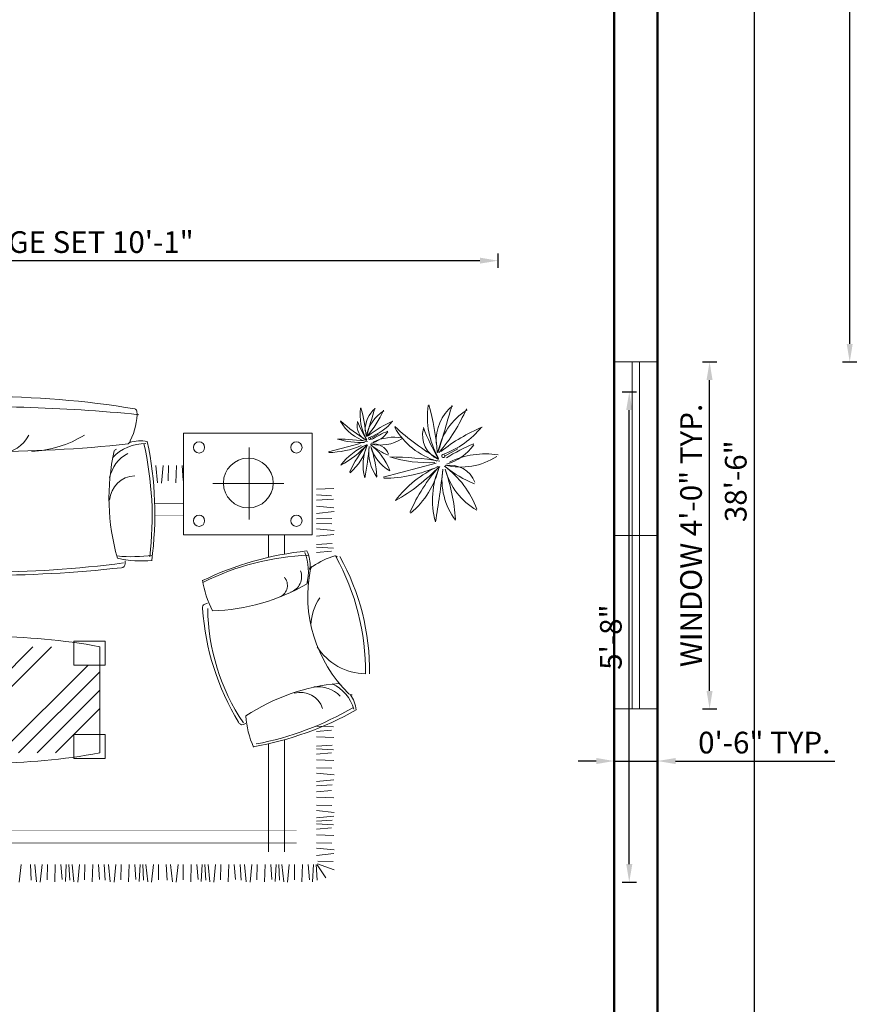
# Model space of a CAD drawing. Units: inches. Extents: x 1961 to 3038, y 800 to 1438.
# Tile 10 of 13: x 2920 to 3038, y 1012 to 1148. Entities that reach past the tile are written whole.
import ezdxf

# ---------------------------------------------------------------- set-up
doc = ezdxf.new("R2010")
doc.units = ezdxf.units.IN
for name, color, linetype, lineweight in [('A-ANNO-DIMS', 2, 'Continuous', 18), ('A-FURN', 8, 'Continuous', 18), ('A-GLAZ', 4, 'Continuous', 18), ('A-WALL', 7, 'Continuous', 50)]:
    doc.layers.add(name, color=color, linetype=linetype, lineweight=lineweight)
doc.styles.get("Standard").update_dxf_attribs({"font": 'arial.ttf'})
doc.dimstyles.new('ISO-25', dxfattribs={"dimtxt": 3, "dimasz": 2.5, "dimexe": 1, "dimexo": 1, "dimtad": 1, "dimdec": 4, "dimlunit": 4, "dimtxsty": 'Standard', "dimcen": 2.5, "dimadec": 0, "dimazin": 0, "dimtfac": 1, "dimtdec": 4, "dimtmove": 0, "dimatfit": 3, "dimfxl": 1, "dimfxlon": 1, "dimarcsym": 0})

# ---------------------------------------------------------------- blocks, each defined once
blk = doc.blocks.new('A$C28C76B35')
for p, q in [((630.8, 2791.1), (1149.7, 2272.2)), ((630.8, 2701.3), (1149.7, 2182.4)), ((630.8, 2431.9), (1059.7, 2003)), ((86.3, 2330.2, -715.1), (0, 2338.9, -715.1)), ((630.8, 2342.1), (1027.2, 1945.7)), ((86.3, 2263.8, -715.1), (1.4, 2255.2, -715.1)), ((86.3, 2285, -715.1), (10.1, 2280.7, -715.1)), ((86.3, 2227.8, -715.1), (0, 2236.5, -715.1)), ((630.8, 2252.3), (937.3, 1945.7)), ((86.3, 2163, -715.1), (1.4, 2165.9, -715.1)), ((86.3, 2201.9, -715.1), (11.5, 2203.3, -715.1)), ((86.3, 2135.7, -715.1), (13, 2129.9, -715.1)), ((630.8, 2162.5), (720.3, 2073)), ((86.3, 2080.9, -715.1), (1.4, 2072.3, -715.1)), ((86.3, 2109.7, -715.1), (2.9, 2114, -715.1)), ((86.3, 2096.8, -715.1), (10.1, 2092.4, -715.1)), ((720.8, 2072.5), (847.5, 1945.7)), ((86.3, 2044.9, -715.1), (0, 2053.6, -715.1)), ((86.3, 2019, -715.1), (11.5, 2020.4, -715.1)), ((86.3, 1980.1, -715.1), (1.4, 1983, -715.1)), ((86.3, 1924.1, -715.1), (10.1, 1919.7, -715.1)), ((86.3, 1952.7, -715.1), (13, 1947, -715.1)), ((1149.7, 1945.7), (630.8, 1945.7)), ((86.3, 1866.9, -715.1), (0, 1875.6, -715.1)), ((86.3, 1902.9, -715.1), (1.4, 1894.3, -715.1)), ((86.3, 1841, -715.1), (11.5, 1842.4, -715.1)), ((86.3, 1802.1, -715.1), (1.4, 1805, -715.1)), ((1569.5, 1821.1, -2545.7), (1554.2, 1821.1, -2545.7)), ((86.3, 1748.8, -715.1), (2.9, 1753.1, -715.1)), ((86.3, 1735.9, -715.1), (10.1, 1731.5, -715.1)), ((86.3, 1774.7, -715.1), (13, 1769, -715.1)), ((86.3, 1684, -715.1), (0, 1692.6, -715.1)), ((86.3, 1720, -715.1), (1.4, 1711.4, -715.1)), ((86.3, 1658.1, -715.1), (11.5, 1659.5, -715.1)), ((2034.4, 1635.7, -715.1), (1948.1, 1644.4, -715.1)), ((2034.4, 1671.7, -715.1), (1949.5, 1663.1, -715.1)), ((86.3, 1599.5, -715.1), (1.4, 1590.9, -715.1)), ((86.3, 1620.7, -715.1), (10.1, 1616.4, -715.1)), ((2034.4, 1609.8, -715.1), (1959.6, 1611.2, -715.1)), ((86.3, 1563.5, -715.1), (0, 1572.2, -715.1)), ((86.3, 1537.6, -715.1), (11.5, 1539, -715.1)), ((2034.4, 1570.9, -715.1), (1949.5, 1573.8, -715.1)), ((2034.4, 1543.6, -715.1), (1961, 1537.8, -715.1)), ((86.3, 1498.7, -715.1), (1.4, 1501.6, -715.1)), ((86.3, 1445.4, -715.1), (2.9, 1449.8, -715.1)), ((86.3, 1471.4, -715.1), (13, 1465.6, -715.1)), ((86.3, 1416.6, -715.1), (1.4, 1408, -715.1)), ((86.3, 1432.5, -715.1), (10.1, 1428.1, -715.1)), ((1361.7, 1420, -2396.1), (1357.7, 1432.5, -2396.1)), ((86.3, 1380.6, -715.1), (0, 1389.3, -715.1)), ((86.3, 1354.7, -715.1), (11.5, 1356.1, -715.1)), ((1945.6, 1046.8, -715.1), (1945.6, 1393.5, -715.1)), ((86.3, 1315.8, -715.1), (1.4, 1318.7, -715.1)), ((86.3, 1259.8, -715.1), (10.1, 1255.4, -715.1)), ((86.3, 1288.5, -715.1), (13, 1282.7, -715.1)), ((86.3, 1202.6, -715.1), (0, 1211.3, -715.1)), ((86.3, 1238.6, -715.1), (1.4, 1230, -715.1)), ((773.9, 1232.5, -2396.1), (769.6, 1245.9, -2396.1)), ((1770.8, 1215.5, -715.1), (2121.9, 1215.5, -715.1)), ((86.3, 1176.7, -715.1), (11.5, 1178.1, -715.1)), ((86.3, 1137.8, -715.1), (1.4, 1140.7, -715.1)), ((86.3, 1110.4, -715.1), (13, 1104.7, -715.1)), ((147.6, 1122, -715.1), (675.9, 1122, -715.1)), ((1585.7, 1122, -715.1), (1695.2, 1122, -715.1)), ((86.3, 1084.5, -715.1), (2.9, 1088.8, -715.1)), ((86.3, 1071.6, -715.1), (10.1, 1067.2, -715.1)), ((86.3, 1019.7, -715.1), (0, 1028.4, -715.1)), ((86.3, 1055.7, -715.1), (1.4, 1047.1, -715.1)), ((147.6, 1043.4, -715.1), (695.7, 1043.4, -715.1)), ((1601.8, 1043.4, -715.1), (1695.2, 1043.4, -715.1)), ((86.3, 993.8, -715.1), (11.5, 995.2, -715.1)), ((86.3, 954.9, -715.1), (1.4, 957.8, -715.1)), ((85.6, 927.5, -715.1), (12.2, 921.8, -715.1)), ((85.6, 901.6, -715.1), (2.1, 905.9, -715.1)), ((85.6, 888.7, -715.1), (9.3, 884.3, -715.1)), ((85.1, 883.2, -715.1), (21.4, 841.3, -715.1)), ((89.1, 881.5, -715.1), (61.1, 800.9, -715.1)), ((102.9, 881.1, -715.1), (101.5, 806.3, -715.1)), ((130.6, 887.5, -715.1), (139.3, 802.6, -715.1)), ((166.6, 887.5, -715.1), (158, 801.2, -715.1)), ((192.5, 887.5, -715.1), (191.1, 812.7, -715.1)), ((231.4, 887.5, -715.1), (228.6, 802.6, -715.1)), ((258.8, 887.5, -715.1), (264.6, 814.1, -715.1)), ((284.7, 887.5, -715.1), (280.4, 804.1, -715.1)), ((297.7, 887.5, -715.1), (302, 811.2, -715.1)), ((313.5, 887.5, -715.1), (322.2, 802.6, -715.1)), ((349.5, 887.5, -715.1), (340.9, 801.2, -715.1)), ((375.4, 887.5, -715.1), (374, 812.7, -715.1)), ((414.3, 887.5, -715.1), (411.5, 802.6, -715.1)), ((441.7, 887.5, -715.1), (447.5, 814.1, -715.1)), ((470.4, 887.5, -715.1), (474.7, 811.2, -715.1)), ((491.5, 887.5, -715.1), (500.2, 802.6, -715.1)), ((532.8, 887.5, -715.1), (524.1, 801.2, -715.1)), ((558.7, 887.5, -715.1), (557.2, 812.7, -715.1)), ((597.6, 887.5, -715.1), (594.7, 802.6, -715.1)), ((624.9, 887.5, -715.1), (630.7, 814.1, -715.1)), ((650.9, 887.5, -715.1), (646.5, 804.1, -715.1)), ((663.8, 887.5, -715.1), (668.1, 811.2, -715.1)), ((708.8, 887.5, -715.1), (705.9, 802.6, -715.1)), ((736.2, 887.5, -715.1), (741.9, 814.1, -715.1)), ((762.1, 887.5, -715.1), (757.8, 804.1, -715.1)), ((1609.5, 887.5, -715.1), (1615.3, 814.1, -715.1)), ((1635.4, 887.5, -715.1), (1631.1, 804.1, -715.1)), ((1648.4, 887.5, -715.1), (1652.7, 811.2, -715.1)), ((1689.1, 887.5, -715.1), (1697.7, 802.6, -715.1)), ((1725.1, 887.5, -715.1), (1716.5, 801.2, -715.1)), ((1751, 887.5, -715.1), (1749.6, 812.7, -715.1)), ((1774.5, 887.5, -715.1), (1775.9, 812.7, -715.1)), ((1800.4, 887.5, -715.1), (1809.1, 801.2, -715.1)), ((1836.4, 887.5, -715.1), (1827.8, 802.6, -715.1)), ((1865.2, 887.5, -715.1), (1869.6, 804.1, -715.1)), ((1891.2, 887.5, -715.1), (1885.4, 814.1, -715.1)), ((1918.5, 887.5, -715.1), (1921.4, 802.6, -715.1)), ((2142.4, 673.8), (2100.9, 828.6)), ((2166.3, 621.8), (2187.1, 584.4)), ((2046.1, 302.6), (1976.9, 560.7)), ((2080.7, 258.1), (2115.3, 195.8))]:
    blk.add_line(p, q)
at = {"const_width": 2.63, "elevation": -715.1}
for points in [[(191.4, 983.4), (191.4, 3592.6)], [(250.4, 983.4), (250.4, 3582.8)], [(1788.8, 1537.3), (1788.8, 1676.7)], [(1847.7, 1537.3), (1847.7, 1677.3)]]:
    blk.add_lwpolyline(points, dxfattribs=at)
for points in [[(604.3, 1919.2), (604.3, 2073), (720.8, 2073), (720.8, 1919.2)], [(1176.1, 1919.2), (1176.1, 2073), (1059.7, 2073), (1059.7, 1919.2)]]:
    blk.add_lwpolyline(points, close=True)
at = {"elevation": -618.7}
blk.add_lwpolyline([(2191.4, 1537.3), (2191.4, 908.3), (1695.2, 908.3), (1695.2, 1537.3)], close=True, dxfattribs=at)
for centre, radius in [((1764.5, 1460.7, -691), 27.3), ((2122.2, 1460.7, -691), 27.3), ((1948.7, 1220.2, -715.1), 121.7), ((1764.5, 984.9, -691), 27.3), ((2122.2, 984.9, -691), 27.3)]:
    blk.add_circle(centre, radius)
for centre, radius, start, end in [((8358.1, 2490.4, -2545.7), 6255.6, 173.16241, 186.27001), ((-1923.8, 2488.5, -2545.7), 4294.1, 350.4205, 10.2522), ((7689.8, 2524.2, -2545.7), 6192.4, 173.65504, 186.34496), ((6606.3, 2502.6, -2545.7), 5092.4, 172.1196, 187.596), ((3583.6, 2486.4), 3001.9, 169.6234, 190.3766), ((-1803.1, 2486.4), 3001.9, 349.6234, 10.3766), ((-5321.3, 2528, -2545.7), 7642.7, 354.19861, 2.64527), ((2254.5, 2435.4, -2545.7), 160, 181.4899, 243.2939), ((2639, 2302.1, -2545.7), 536, 182.4337, 211.6473), ((1874, 836.9, -2545.7), 1063.9, 77.442, 105.9291), ((1857.7, 1771.4, -2545.7), 126.3, 1.587, 86.7541), ((1939.9, 1727.6, -2545.7), 173.3, 28.0169, 78.7258), ((1922.8, 1724.7, -2545.7), 218.5, 358.8733, 46.7696), ((1977.4, 1755.8, -2545.7), 175.1, 38.5221, 43.0547), ((1554.2, 1839.9, -2545.7), 18.8, 180, 270), ((2051, 1743.8, -2545.7), 482.9, 166.0947, 186.4886), ((2327.1, 1788.6, -2545.7), 738, 174.4394, 187.8276), ((2156.7, 1815.6, -2545.7), 18.8, 206.5221, 265.2757), ((1979.2, 1747.6, -2545.7), 175.5, 348.8784, 17.2062), ((2289.3, 2051.1, -2545.7), 287.4, 242.1884, 272.3768), ((1782.8, 3287.1, -2545.7), 1597.2, 263.0352, 282.9689), ((2293, 1780.9, -2545.7), 18.8, 295.7033, 338.2144), ((1798.6, 3371.1, -2545.7), 1694.4, 262.251, 282.0202), ((1421.4, 211.6, -2396.1), 1235.1, 93.9636, 121.2426), ((1534.9, 1000.6, -2396.1), 446.8, 97.6899, 118.0066), ((1341.3, 1427.3, -2396.1), 17.3, 17.6031, 107.6031), ((92, 775.7, -2396.1), 1533.4, 5.9051, 25.8197), ((1349.7, 392.7, -2396.1), 1025.7, 90.7293, 123.8646), ((2301.4, 1423.8, -2396.1), 976.9, 181.674, 210.1612), ((361.3, 881.6, -2396.1), 1235.6, 2.0942, 26.8169), ((786.1, 1251.1, -2396.1), 17.3, 107.6031, 197.6031), ((840, 789.6, -2396.1), 443.4, 93.6978, 114.0917), ((-3, 692.6, -2396.1), 976.9, 5.0451, 33.5322), ((2194.2, 1462.4, -2396.1), 1556, 189.8541, 209.6233), ((2116.3, 1452.9, -2396.1), 1466.7, 190.6383, 210.572), ((1448.6, 1090.6, -2396.1), 61.6, 206.9826, 310.1527), ((1491.3, 1039.3, -2396.1), 79.7, 198.6132, 291.0431), ((810.5, 966.5, -2396.1), 116, 289.1901, 14.3572), ((1395.4, 264.8, -2396.1), 664.6, 78.3859, 135.6519), ((1248.4, 666, -2396.1), 248.4, 55.5581, 88.0156), ((1516.4, 1184.4, -2396.1), 257.8, 256.0323, 291.3332), ((1525.9, 1078.1, -2396.1), 160.8, 244.5484, 249.0811), ((1523.3, 904.5, -2396.1), 17.3, 22.3274, 81.0811), ((1525.7, 898.9, -2396.1), 17.3, 15.6232, 78.3859), ((1525.7, 898.9, -2396.1), 17.3, 15.0401, 75.224), ((1542.4, 1100.2, -2396.1), 182.8, 267.5646, 294.1582), ((794.9, 882.3, -2396.1), 159.2, 315.62, 6.3289), ((1301.9, 643.6, -2396.1), 284.4, 122.5868, 179.1326), ((1209.3, 676.9, -2396.1), 402.9, 17.4821, 34.236), ((2490.7, 828.5), 392.8, 180.242, 204.0498), ((787.7, 896.5, -2396.1), 200.7, 286.4764, 334.3727), ((830, 857.3, -2396.1), 160.8, 326.1252, 330.6578), ((1030.3, 1799.9, -2396.1), 1152, 269.3654, 299.0389), ((1030.3, 1779.7, -2396.1), 1152, 269.3654, 299.0389), ((1576.3, 798.2, -2396.1), 17.3, 310.9353, 358.9668), ((1576.4, 798.3, -2396.1), 17.3, 311.6789, 353.9346), ((2539.7, 670.2), 393.1, 163.2117, 182.6473), ((1251.8, 784.4), 911.5, 350.7455, 359.9594), ((2356.2, 583.9), 214.1, 119.9306, 162.9527), ((2820.5, 249.3), 770.3, 137.5232, 149.4062), ((823.4, 853.5, -2396.1), 161.2, 276.4815, 304.8093), ((932.2, 717, -2396.1), 17.3, 134.1252, 192.8788), ((2193.4, 886.6), 254.1, 220.0008, 256.4192), ((1789.6, 246.8), 523.1, 48.6584, 66.0848), ((2496, 1021.9), 525.7, 208.9098, 226.6574), ((1839.9, 509.6), 324.1, 24.3367, 52.802), ((2227.4, 610.2), 78, 75.9187, 156.4457), ((2439.6, 184.8), 536, 110.7855, 121.5789), ((2281.3, 432.8), 241.2, 82.0464, 119.2724), ((2037.5, 425.8), 233.5, 65.269, 105.9092), ((2355.8, 2841.9), 2224.7, 260.1053, 264.1165), ((2096.3, 434.8), 196.4, 81.2259, 127.0636), ((2166.3, 627.3), 4.79, 19.6875, 308.9221), ((2417.3, 717.1), 261.8, 199.6875, 230.5302), ((2143.5, 460.6), 185.3, 31.6153, 80.1372), ((4441.4, 8102.1), 7795.6, 253.10003, 254.16808), ((2127.1, 1324.7), 681.5, 274.1768, 286.1059), ((2516.1, 1038.6), 523.8, 229.6107, 246.1427), ((1778.5, 316.9), 511.5, 22.5722, 38.3507), ((2209.8, 513.7), 135, 40.0083, 92.7048), ((1935.5, 1183.5), 593.7, 274.3837, 288.8918), ((2179.5, 430.3), 198.3, 105.1243, 150.0802), ((1910.9, 794), 282.9, 290.6384, 322.9635), ((2414.3, 399.4), 356.9, 141.4571, 157.4335), ((2061.4, 607.5), 78, 290.8411, 10.5336), ((2328, 575.4), 194, 166.1764, 212.74), ((2283.1, 657.2), 145.8, 195.5054, 234.7561), ((1936.1, 505.7), 236.4, 350.5683, 26.0168), ((1741.8, 350.4), 497, 22.1939, 32.6137), ((2626.6, 560.5), 654.7, 180.242, 204.0498), ((2630.1, 924.9), 876.1, 208.9098, 226.6574), ((1536.6, 71.1), 540.2, 24.3367, 52.802), ((2703.1, 338.8), 655.2, 163.2117, 182.6473), ((556.6, 529.1), 1519.2, 350.7455, 359.9594), ((2397.2, 195), 356.9, 119.9306, 162.9527), ((3171, -362.7), 1283.9, 137.5232, 149.4062), ((2125.8, 699.4), 423.5, 220.0008, 256.4192), ((1452.8, -366.8), 871.9, 48.6584, 66.0848), ((2182.6, 238.8), 130, 75.9187, 156.4457), ((2536.1, -470.2), 893.3, 110.7855, 121.5789), ((2272.3, -56.9), 401.9, 82.0464, 119.2724), ((2015.3, 1429.5), 1135.9, 274.1768, 286.1059), ((1866, -68.6), 389.1, 65.269, 105.9092), ((2396.5, 3958.2), 3707.8, 260.1053, 264.1165), ((2042.6, -10.6), 308.8, 31.6153, 80.1372), ((5872.5, 12725.3), 12992.7, 253.10003, 254.16808), ((2153.1, 77.9), 225, 40.0083, 92.7048), ((1964, -53.5), 327.3, 81.2259, 127.0636), ((1696, 1194.3), 989.5, 274.3837, 288.8918), ((2102.6, -61), 330.5, 105.1243, 150.0802), ((1655, 545), 471.4, 290.6384, 322.9635), ((2494, -112.6), 594.9, 141.4571, 157.4335), ((1905.9, 234.3), 130.1, 290.8411, 10.5336), ((2350.2, 180.8), 323.4, 166.1764, 212.74), ((2275.4, 317.2), 243.1, 195.5054, 234.7561), ((1373.2, -194.2), 828.3, 22.1939, 32.6137), ((2080.6, 267.3), 7.98, 19.6875, 308.9221), ((2499, 417), 436.3, 199.6875, 230.5302), ((2663.7, 952.7), 873.1, 229.6107, 246.1427), ((1434.4, -250.1), 852.5, 22.5722, 38.3507), ((1697, 64.6), 393.9, 350.5683, 26.0168)]:
    blk.add_arc(centre, radius, start, end)
blk = doc.blocks.new('*D26')
at = {"layer": 'A-ANNO-DIMS', "color": 0, "lineweight": -2, "transparency": 16777216}
for p, q in [((3021.14, 1314.92), (3023.14, 1314.92)), ((3022.14, 1312.42), (3022.14, 855.42)), ((3021.14, 852.92), (3023.14, 852.92))]:
    blk.add_line(p, q, dxfattribs=at)
at = {"layer": 'A-ANNO-DIMS', "color": 0, "transparency": 16777216}
for points in [[(3021.72, 1312.42), (3022.55, 1312.42), (3022.14, 1314.92)], [(3021.72, 855.42), (3022.55, 855.42), (3022.14, 852.92)]]:
    blk.add_solid(points, dxfattribs=at)
at = {"layer": 'Defpoints', "color": 0, "transparency": 16777216}
for p in [(3008.77, 1314.92), (3008.77, 852.92), (3022.14, 852.92)]:
    blk.add_point(p, dxfattribs=at)
at = {"layer": 'A-ANNO-DIMS', "color": 0, "transparency": 16777216, "insert": (3019.98, 1083.92), "char_height": 3, "attachment_point": 5, "rotation": 90}
blk.add_mtext('38\'-6"', dxfattribs=at)
blk = doc.blocks.new('WIN-48IN-MULLION')
for p, q in [((6, 48), (0, 48)), ((2.5, 48), (2.5, 0)), ((3.5, 48), (3.5, 0)), ((6, 24), (0, 24)), ((6, 0), (0, 0))]:
    blk.add_line(p, q)
blk = doc.blocks.new('*D45')
at = {"layer": 'A-ANNO-DIMS', "color": 0, "lineweight": -2, "transparency": 16777216}
for p, q in [((3014.97, 1100.42), (3016.97, 1100.42)), ((3015.97, 1054.92), (3015.97, 1097.92)), ((3014.97, 1052.42), (3016.97, 1052.42))]:
    blk.add_line(p, q, dxfattribs=at)
at = {"layer": 'A-ANNO-DIMS', "color": 0, "transparency": 16777216}
for points in [[(3015.55, 1097.92), (3016.38, 1097.92), (3015.97, 1100.42)], [(3015.55, 1054.92), (3016.38, 1054.92), (3015.97, 1052.42)]]:
    blk.add_solid(points, dxfattribs=at)
at = {"layer": 'Defpoints', "color": 0, "transparency": 16777216}
for p in [(3008.77, 1100.42), (3015.97, 1100.42), (3008.77, 1052.42)]:
    blk.add_point(p, dxfattribs=at)
at = {"layer": 'A-ANNO-DIMS', "color": 0, "transparency": 16777216, "insert": (3013.79, 1076.42), "char_height": 3, "attachment_point": 5, "rotation": 90}
blk.add_mtext('WINDOW 4\'-0" TYP.', dxfattribs=at)
blk = doc.blocks.new('*D46')
at = {"layer": 'A-ANNO-DIMS', "color": 0, "lineweight": -2, "transparency": 16777216}
for p, q in [((3002.77, 1046.22), (3002.77, 1044.22)), ((3008.77, 1046.22), (3008.77, 1044.22)), ((3000.27, 1045.22), (2997.77, 1045.22)), ((3002.77, 1045.22), (3008.77, 1045.22)), ((3011.27, 1045.22), (3033.3, 1045.22))]:
    blk.add_line(p, q, dxfattribs=at)
at = {"layer": 'A-ANNO-DIMS', "color": 0, "transparency": 16777216}
for points in [[(3000.27, 1045.64), (3000.27, 1044.8), (3002.77, 1045.22)], [(3011.27, 1045.64), (3011.27, 1044.8), (3008.77, 1045.22)]]:
    blk.add_solid(points, dxfattribs=at)
at = {"layer": 'Defpoints', "color": 0, "transparency": 16777216}
for p in [(3002.77, 1052.42), (3008.77, 1052.42), (3008.77, 1045.22)]:
    blk.add_point(p, dxfattribs=at)
at = {"layer": 'A-ANNO-DIMS', "color": 0, "transparency": 16777216, "insert": (3023.54, 1047.38), "char_height": 3, "attachment_point": 5}
blk.add_mtext('0\'-6" TYP.', dxfattribs=at)
blk = doc.blocks.new('*D63')
at = {"layer": 'A-ANNO-DIMS', "color": 0, "lineweight": -2, "transparency": 16777216}
for p, q in [((2865.57, 1113.43), (2865.57, 1115.43)), ((2986.68, 1113.43), (2986.68, 1115.43)), ((2984.18, 1114.43), (2868.07, 1114.43))]:
    blk.add_line(p, q, dxfattribs=at)
at = {"layer": 'A-ANNO-DIMS', "color": 0, "transparency": 16777216}
for points in [[(2868.07, 1114.85), (2868.07, 1114.02), (2865.57, 1114.43)], [(2984.18, 1114.85), (2984.18, 1114.02), (2986.68, 1114.43)]]:
    blk.add_solid(points, dxfattribs=at)
at = {"layer": 'Defpoints', "color": 0, "transparency": 16777216}
for p in [(2865.57, 1114.43), (2865.57, 1096.27), (2986.68, 1096.27)]:
    blk.add_point(p, dxfattribs=at)
at = {"layer": 'A-ANNO-DIMS', "color": 0, "transparency": 16777216, "insert": (2926.13, 1116.61), "char_height": 3, "attachment_point": 5}
blk.add_mtext('LOUNGE SET 10\'-1"', dxfattribs=at)
blk = doc.blocks.new('*D64')
at = {"layer": 'A-ANNO-DIMS', "color": 0, "lineweight": -2, "transparency": 16777216}
for p, q in [((3003.85, 1096.27), (3005.85, 1096.27)), ((3004.85, 1030.96), (3004.85, 1093.77)), ((3003.85, 1028.46), (3005.85, 1028.46))]:
    blk.add_line(p, q, dxfattribs=at)
at = {"layer": 'A-ANNO-DIMS', "color": 0, "transparency": 16777216}
for points in [[(3004.43, 1093.77), (3005.27, 1093.77), (3004.85, 1096.27)], [(3004.43, 1030.96), (3005.27, 1030.96), (3004.85, 1028.46)]]:
    blk.add_solid(points, dxfattribs=at)
at = {"layer": 'Defpoints', "color": 0, "transparency": 16777216}
for p in [(2986.68, 1096.27), (3004.85, 1096.27), (2986.68, 1028.46)]:
    blk.add_point(p, dxfattribs=at)
at = {"layer": 'A-ANNO-DIMS', "color": 0, "transparency": 16777216, "insert": (3002.69, 1062.36), "char_height": 3, "attachment_point": 5, "rotation": 90}
blk.add_mtext('5\'-8"', dxfattribs=at)
blk = doc.blocks.new('*D83')
at = {"layer": 'A-ANNO-DIMS', "color": 0, "lineweight": -2, "transparency": 16777216}
for p, q in [((3034.37, 1314.92), (3036.37, 1314.92)), ((3035.37, 1102.92), (3035.37, 1312.42)), ((3034.37, 1100.42), (3036.37, 1100.42))]:
    blk.add_line(p, q, dxfattribs=at)
at = {"layer": 'A-ANNO-DIMS', "color": 0, "transparency": 16777216}
for points in [[(3034.95, 1312.42), (3035.78, 1312.42), (3035.37, 1314.92)], [(3034.95, 1102.92), (3035.78, 1102.92), (3035.37, 1100.42)]]:
    blk.add_solid(points, dxfattribs=at)
at = {"layer": 'Defpoints', "color": 0, "transparency": 16777216}
for p in [(3008.77, 1314.92), (3035.37, 1314.92), (3008.77, 1100.42)]:
    blk.add_point(p, dxfattribs=at)
at = {"layer": 'A-ANNO-DIMS', "color": 0, "transparency": 16777216, "insert": (3033.19, 1207.67), "char_height": 3, "attachment_point": 5, "rotation": 90}
blk.add_mtext('17\'-10 1/2"', dxfattribs=at)

msp = doc.modelspace()

# ---------------------------------------------------------------- linework, layer by layer
at = {"layer": 'A-WALL'}
for p, q in [((3008.76803, 852.91975), (3008.76803, 1314.91975)), ((3002.76803, 975.41975), (3002.76803, 1160.41975))]:
    msp.add_line(p, q, dxfattribs=at)

# ---------------------------------------------------------------- block references
at = {"layer": 'A-FURN', "xscale": 0.0283328092017671, "yscale": 0.0283328092017671, "zscale": 0.0283328092017671, "rotation": 90}
msp.add_blockref('A$C28C76B35', (2986.6849, 1028.46179, 88.65501), dxfattribs=at)
at = {"layer": 'A-GLAZ'}
msp.add_blockref('WIN-48IN-MULLION', (3002.768, 1052.42), dxfattribs=at)

# ---------------------------------------------------------------- dimensions: what is measured, and where the dimension line sits
at = {"layer": 'A-ANNO-DIMS'}
for base, p1, p2, override, picture, middle in [((3022.1353, 852.91975), (3008.76803, 1314.91975), (3008.76803, 852.91975), {"dimclrd": 0, "dimclre": 0, "dimclrt": 0}, '*D26', (3019.97756, 1083.91975)), ((3035.36803, 1314.91975), (3008.76803, 1100.41975), (3008.76803, 1314.91975), {"dimdec": 1, "dimlfac": 1, "dimrnd": 0, "dimzin": 1, "dimdsep": 46, "dimlunit": 4, "dimfrac": 2}, '*D83', (3033.19187, 1207.66975)), ((3004.85164, 1096.26631), (2986.6849, 1028.46178), (2986.6849, 1096.26631), {"dimdec": 1, "dimlfac": 1, "dimrnd": 0, "dimzin": 1, "dimdsep": 46, "dimlunit": 4, "dimfrac": 2}, '*D64', (3002.69492, 1062.36404))]:
    dim = msp.add_linear_dim(base=base, p1=p1, p2=p2, angle=90, dimstyle='ISO-25', override=override, dxfattribs=at)
    dim.commit()
    dim.dimension.update_dxf_attribs({"geometry": picture, "text_midpoint": middle})
for base, p1, p2, angle, text, picture, middle in [((2865.57325, 1114.43305), (2986.6849, 1096.26631), (2865.57325, 1096.26631), 180, 'LOUNGE SET <>', '*D63', (2926.12907, 1116.61024)), ((3015.96803, 1100.41975), (3008.76803, 1052.41975), (3008.76803, 1100.41975), 90, 'WINDOW <> TYP.', '*D45', (3013.79085, 1076.41975))]:
    dim = msp.add_linear_dim(base=base, p1=p1, p2=p2, angle=angle, text=text, dimstyle='ISO-25', override={"dimdec": 1, "dimlfac": 1, "dimrnd": 0, "dimzin": 1, "dimdsep": 46, "dimlunit": 4, "dimfrac": 2}, dxfattribs=at)
    dim.commit()
    dim.dimension.update_dxf_attribs({"geometry": picture, "text_midpoint": middle})
dim = msp.add_linear_dim(base=(3008.76803, 1045.21975), p1=(3002.76803, 1052.41975), p2=(3008.76803, 1052.41975), text='<> TYP.', dimstyle='ISO-25', override={"dimdec": 1, "dimlfac": 1, "dimrnd": 0, "dimzin": 1, "dimdsep": 46, "dimlunit": 4, "dimfrac": 2}, dxfattribs=at)
dim.commit()
dim.dimension.update_dxf_attribs({"geometry": '*D46', "text_midpoint": (3023.53628, 1047.37647)})

doc.saveas('drawing.dxf')
